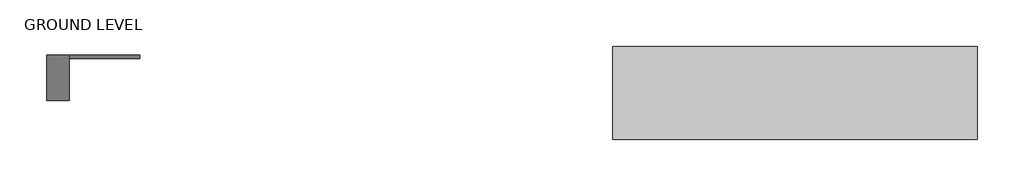
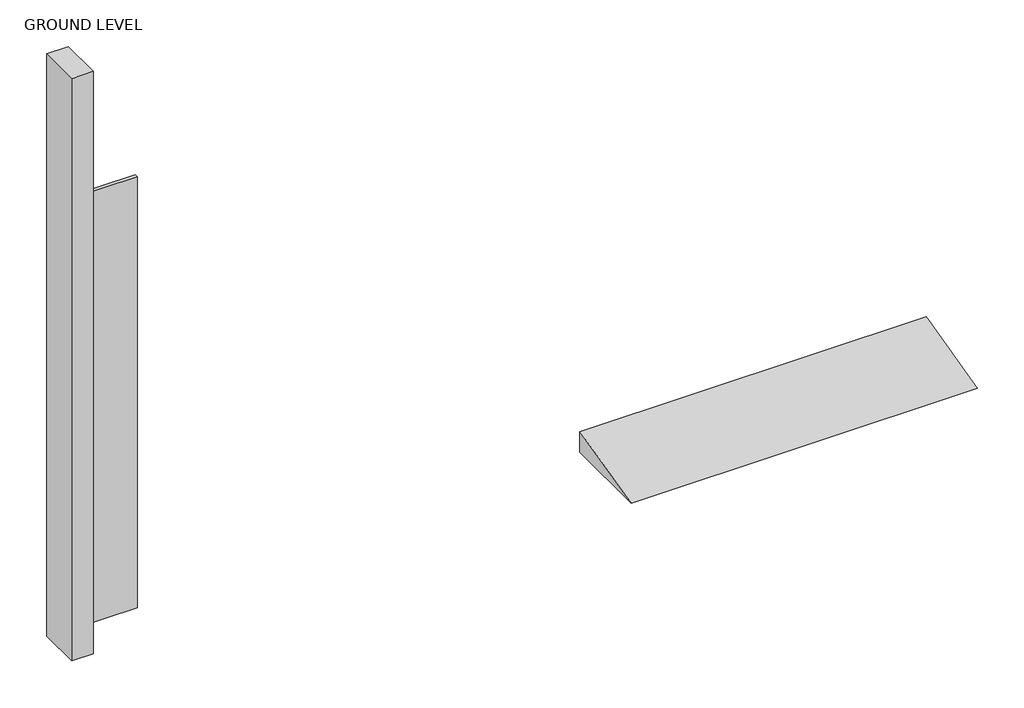
# One storey, incomplete: 3 proxies.
"""IFC4 building model written with IfcOpenShell, lengths in millimetres."""

from ifc_helpers import new_model, si_unit, origin, place, context, project, spatial, transform, mapped, element, save
from components import generic_models_26_generic_models_26_2c916a27, generic_models_3_generic_models_3_72a9eea6, generic_models_4_generic_models_4_e71d7c83

model = new_model("IFC4")

# Units and contexts
model_context = context("Model", 3, world=origin())
ifc_project = project(units=[si_unit("LENGTHUNIT", "METRE", prefix="MILLI")], contexts=[model_context])

# Site, building, storey
site = spatial("IfcSite", under=ifc_project)
building = spatial("IfcBuilding", under=site)
storey = spatial("IfcBuildingStorey", under=building, Name="GROUND LEVEL", Elevation=0.0)

# Proxies
placement = place(None, origin())
generic_models_26_generic_models_26_shape = generic_models_26_generic_models_26_2c916a27(model_context)
element("IfcBuildingElementProxy", 1, Name="Generic Models 26 : Generic Models 26", ObjectType="Generic Models 26 : Generic Models 26", at=placement, inside=storey, context=model_context, shape_type="MappedRepresentation", body=[
    mapped(generic_models_26_generic_models_26_shape, transform((0.0, 0.0, 0.0), x_axis=(1.0, 0.0, 0.0), y_axis=(0.0, 1.0, 0.0), z_axis=(0.0, 0.0, 1.0))),
])
generic_models_3_generic_models_3_shape = generic_models_3_generic_models_3_72a9eea6(model_context)
element("IfcBuildingElementProxy", 2, Name="Generic Models 3 : Generic Models 3", ObjectType="Generic Models 3 : Generic Models 3", at=placement, inside=storey, context=model_context, shape_type="MappedRepresentation", body=[
    mapped(generic_models_3_generic_models_3_shape, transform((0.0, 0.0, 0.0), x_axis=(1.0, 0.0, 0.0), y_axis=(0.0, 1.0, 0.0), z_axis=(0.0, 0.0, 1.0))),
])
generic_models_4_generic_models_4_shape = generic_models_4_generic_models_4_e71d7c83(model_context)
element("IfcBuildingElementProxy", 3, Name="Generic Models 4 : Generic Models 4", ObjectType="Generic Models 4 : Generic Models 4", at=placement, inside=storey, context=model_context, shape_type="MappedRepresentation", body=[
    mapped(generic_models_4_generic_models_4_shape, transform((0.0, 0.0, 0.0), x_axis=(1.0, 0.0, 0.0), y_axis=(0.0, 1.0, 0.0), z_axis=(0.0, 0.0, 1.0))),
])

save(model, "model.ifc")

# Revit data of these elements
# Element 1 (IfcBuildingElementProxy, "Generic Models 26 : Generic Models 26")
#   Phase Created = New Construction
#   Materials on its faces: "Concrete, Cast-in-Place gray"
# Element 2 (IfcBuildingElementProxy, "Generic Models 3 : Generic Models 3")
#   Phase Created = New Construction
#   Materials on its faces: "ESPRESSO"
# Element 3 (IfcBuildingElementProxy, "Generic Models 4 : Generic Models 4")
#   Phase Created = New Construction
#   Materials on its faces: "SAND STONE BEIGE CLADDING"
# Materials
#   "Concrete, Cast-in-Place gray": class "Concrete", colour RGB 192 192 192, transparency 0, Description = "Cast-in-place concrete", Cost = 0
#   "ESPRESSO": class "Generic", colour RGB 120 120 120, transparency 0, Cost = 0
#   "SAND STONE BEIGE CLADDING": class "Generic", colour RGB 120 120 120, transparency 0, Cost = 0
